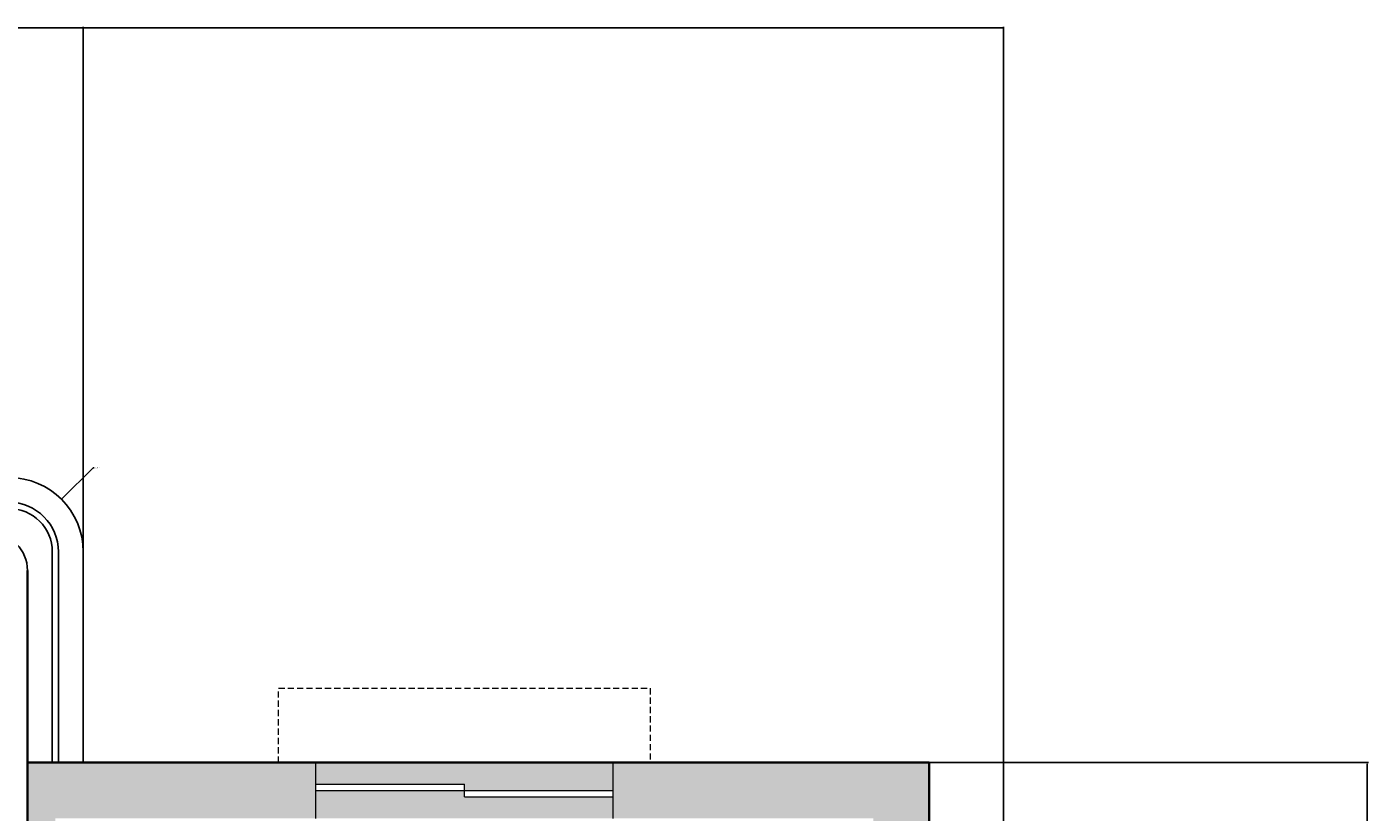
# Model space of a CAD drawing. Units: inches. Extents: x 1693 to 2974, y 2201 to 2965.
# Tile 24 of 24: x 2757 to 2973, y 2838 to 2965. Entities that reach past the tile are written whole.
import ezdxf

# ---------------------------------------------------------------- set-up
doc = ezdxf.new("R2010")
doc.units = ezdxf.units.IN
doc.header["$LTSCALE"] = 2
doc.header["$MEASUREMENT"] = 0
doc.linetypes.add('HIDDEN', pattern=[0.375, 0.25, -0.125])
for name, color, linetype, lineweight in [('A-ANNO-DIMS', 2, 'Continuous', 18), ('A-FLOR-RAIL', 7, 'Continuous', 25), ('A-GLAZ', 4, 'Continuous', 18), ('A-GLAZ-OVHD', 8, 'HIDDEN', 13), ('A-WALL', 7, 'Continuous', 35)]:
    doc.layers.add(name, color=color, linetype=linetype, lineweight=lineweight)
doc.layers.add('A-GLAZ-PATT', color=141, linetype='Continuous', lineweight=13, true_color=0xadddf7)
doc.layers.add('A-WALL-PATT', color=251, linetype='Continuous', lineweight=13, true_color=0x636466)
doc.styles.get("Standard").update_dxf_attribs({"font": 'arial.ttf'})
doc.dimstyles.get("Standard").update_dxf_attribs({"dimtxt": 0.18, "dimasz": 0.18, "dimexe": 0.18, "dimexo": 0.0625, "dimgap": 0.09, "dimtad": 0, "dimtih": 1, "dimtoh": 1, "dimdec": 1, "dimzin": 0, "dimdsep": 46, "dimlunit": 3, "dimtxsty": 'Standard', "dimcen": 0.09, "dimadec": 0, "dimazin": 0, "dimtfac": 1, "dimtdec": 1, "dimtofl": 0, "dimtmove": 0, "dimatfit": 3, "dimfxl": 1, "dimtolj": 1, "dimtzin": 0, "dimarcsym": 0})

# ---------------------------------------------------------------- blocks, each defined once
blk = doc.blocks.new('*D81')
at = {"layer": 'A-ANNO-DIMS', "color": 0, "lineweight": -2, "ltscale": 2, "transparency": 16777216}
for p, q in [((1752.34, 2553.91), (1752.34, 2964.96)), ((1752.52, 2964.78), (2332.94, 2964.78)), ((2914.06, 2964.78), (2333.64, 2964.78)), ((2914.24, 2754.97), (2914.24, 2964.96))]:
    blk.add_line(p, q, dxfattribs=at)
at = {"layer": 'A-ANNO-DIMS', "color": 0, "ltscale": 2, "transparency": 16777216}
for points in [[(1752.52, 2964.81), (1752.52, 2964.75), (1752.34, 2964.78)], [(2914.06, 2964.81), (2914.06, 2964.75), (2914.24, 2964.78)]]:
    blk.add_solid(points, dxfattribs=at)
at = {"layer": 'Defpoints', "color": 0, "ltscale": 2, "transparency": 16777216}
for p in [(2914.24, 2964.78), (2914.24, 2754.9), (1752.34, 2553.84)]:
    blk.add_point(p, dxfattribs=at)
at = {"layer": 'A-ANNO-DIMS', "color": 0, "ltscale": 2, "transparency": 16777216, "insert": (2333.29, 2964.78), "char_height": 0.18, "attachment_point": 5}
blk.add_mtext('\\A1;1162', dxfattribs=at)
blk = doc.blocks.new('*D87')
at = {"layer": 'A-ANNO-DIMS', "color": 0, "lineweight": -2, "ltscale": 2, "transparency": 16777216}
for p, q in [((2902.3, 2846.25), (2973.12, 2846.25)), ((2972.94, 2846.07), (2972.94, 2590.69)), ((2972.94, 2334.93), (2972.94, 2590.32)), ((2902.3, 2334.75), (2973.12, 2334.75))]:
    blk.add_line(p, q, dxfattribs=at)
at = {"layer": 'A-ANNO-DIMS', "color": 0, "ltscale": 2, "transparency": 16777216}
for points in [[(2972.91, 2846.07), (2972.97, 2846.07), (2972.94, 2846.25)], [(2972.91, 2334.93), (2972.97, 2334.93), (2972.94, 2334.75)]]:
    blk.add_solid(points, dxfattribs=at)
at = {"layer": 'Defpoints', "color": 0, "ltscale": 2, "transparency": 16777216}
for p in [(2902.24, 2846.25), (2972.94, 2846.25), (2902.24, 2334.75)]:
    blk.add_point(p, dxfattribs=at)
at = {"layer": 'A-ANNO-DIMS', "color": 0, "ltscale": 2, "transparency": 16777216, "insert": (2972.94, 2590.5), "char_height": 0.18, "attachment_point": 5}
blk.add_mtext('\\A1;511.5', dxfattribs=at)
blk = doc.blocks.new('*D100')
at = {"layer": 'A-ANNO-DIMS', "color": 0, "lineweight": -2, "ltscale": 2, "transparency": 16777216}
for p, q in [((2615.74, 2906.14), (2615.74, 2964.96)), ((2615.92, 2964.78), (2690.46, 2964.78)), ((2765.56, 2964.78), (2691.02, 2964.78)), ((2765.74, 2880.32), (2765.74, 2964.96))]:
    blk.add_line(p, q, dxfattribs=at)
at = {"layer": 'A-ANNO-DIMS', "color": 0, "ltscale": 2, "transparency": 16777216}
for points in [[(2615.92, 2964.81), (2615.92, 2964.75), (2615.74, 2964.78)], [(2765.56, 2964.81), (2765.56, 2964.75), (2765.74, 2964.78)]]:
    blk.add_solid(points, dxfattribs=at)
at = {"layer": 'Defpoints', "color": 0, "ltscale": 2, "transparency": 16777216}
for p in [(2765.74, 2964.78), (2615.74, 2906.08), (2765.74, 2880.25)]:
    blk.add_point(p, dxfattribs=at)
at = {"layer": 'A-ANNO-DIMS', "color": 0, "ltscale": 2, "transparency": 16777216, "insert": (2690.74, 2964.78), "char_height": 0.18, "attachment_point": 5}
blk.add_mtext('\\A1;150', dxfattribs=at)
blk = doc.blocks.new('*D112')
at = {"layer": 'A-ANNO-DIMS', "color": 0, "lineweight": -2, "ltscale": 2, "transparency": 16777216}
for p, q in [((2767.31, 2893.83), (2762.35, 2888.87)), ((2767.49, 2893.83), (2767.31, 2893.83)), ((2753.65, 2880.25), (2753.83, 2880.25)), ((2753.74, 2880.16), (2753.74, 2880.34))]:
    blk.add_line(p, q, dxfattribs=at)
at = {"layer": 'A-ANNO-DIMS', "color": 0, "ltscale": 2, "transparency": 16777216}
blk.add_solid([(2762.33, 2888.89), (2762.37, 2888.85), (2762.22, 2888.74)], dxfattribs=at)
at = {"layer": 'Defpoints', "color": 0, "ltscale": 2, "transparency": 16777216}
for p in [(2762.22, 2888.74), (2753.74, 2880.25)]:
    blk.add_point(p, dxfattribs=at)
at = {"layer": 'A-ANNO-DIMS', "color": 0, "ltscale": 2, "transparency": 16777216, "insert": (2767.99, 2893.83), "char_height": 0.18, "attachment_point": 5}
blk.add_mtext('\\A1;2X R12', dxfattribs=at)

msp = doc.modelspace()

# ---------------------------------------------------------------- hatches: boundary and pattern name
at = {"layer": 'A-GLAZ-PATT', "ltscale": 2}
h = msp.add_hatch(color=256, dxfattribs=at)
h.dxf.hatch_style = 1
h.paths.add_polyline_path([(2656.9702, 2338.2547), (2632.9702, 2338.2547), (2632.9702, 2339.2547), (2608.9702, 2339.2547), (2608.9702, 2334.7547), (2656.9702, 2334.7547)])
h.paths.add_polyline_path([(2656.9702, 2343.7547), (2608.9702, 2343.7547), (2608.9702, 2340.2547), (2632.9702, 2340.2547), (2632.9702, 2339.2547), (2656.9702, 2339.2547)])
h.paths.add_polyline_path([(2775.7544, 2338.2547), (2751.7544, 2338.2547), (2751.7544, 2334.7547), (2775.7544, 2334.7547)])
h.paths.add_polyline_path([(2775.7544, 2343.7547), (2751.7544, 2343.7547), (2751.7544, 2340.2547), (2775.7544, 2340.2547)])
h.paths.add_polyline_path([(2897.7363, 2568.7999), (2893.2363, 2568.7999), (2893.2363, 2520.7999), (2896.7363, 2520.7999), (2896.7363, 2544.7999), (2897.7363, 2544.7999)])
h.paths.add_polyline_path([(2902.2363, 2568.7999), (2898.7363, 2568.7999), (2898.7363, 2544.7999), (2897.7363, 2544.7999), (2897.7363, 2520.7999), (2902.2363, 2520.7999)])
h.paths.add_polyline_path([(2902.2363, 2637.7547), (2898.7363, 2637.7547), (2898.7363, 2613.7547), (2902.2363, 2613.7547)])
h.paths.add_polyline_path([(2896.7363, 2637.7547), (2893.2363, 2637.7547), (2893.2363, 2613.7547), (2896.7363, 2613.7547)])
h.paths.add_polyline_path([(2902.2363, 2748.903), (2899.0477, 2748.903), (2899.0477, 2724.903), (2898.0477, 2724.903), (2898.0477, 2700.903), (2902.2363, 2700.903)])
h.paths.add_polyline_path([(2898.0477, 2748.903), (2893.2363, 2748.903), (2893.2363, 2700.903), (2897.0477, 2700.903), (2897.0477, 2724.903), (2898.0477, 2724.903)])
h.paths.add_polyline_path([(2851.2363, 2846.2547), (2803.2363, 2846.2547), (2803.2363, 2842.7547), (2827.2363, 2842.7547), (2827.2363, 2841.7547), (2851.2363, 2841.7547)])
h.paths.add_polyline_path([(2851.2363, 2840.7547), (2827.2363, 2840.7547), (2827.2363, 2841.7547), (2803.2363, 2841.7547), (2803.2363, 2837.2547), (2851.2363, 2837.2547)])
h.paths.add_polyline_path([(2578.2363, 2846.2547), (2530.2363, 2846.2547), (2530.2363, 2842.7547), (2554.2363, 2842.7547), (2554.2363, 2841.7547), (2578.2363, 2841.7547)])
h.paths.add_polyline_path([(2578.2363, 2840.7547), (2554.2363, 2840.7547), (2554.2363, 2841.7547), (2530.2363, 2841.7547), (2530.2363, 2837.2547), (2578.2363, 2837.2547)])
h.paths.add_polyline_path([(2732.7363, 2812.7547), (2705.1363, 2812.7547), (2705.1363, 2811.7547), (2676.3363, 2811.7547), (2676.3363, 2812.7547), (2648.7363, 2812.7547), (2648.7363, 2808.2547), (2732.7363, 2808.2547)])
h.paths.add_polyline_path([(2732.7363, 2817.2547), (2648.7363, 2817.2547), (2648.7363, 2813.7547), (2676.3363, 2813.7547), (2676.3363, 2812.7547), (2705.1363, 2812.7547), (2705.1363, 2813.7547), (2732.7363, 2813.7547)])
h.paths.add_polyline_path([(2488.2363, 2695.8203), (2484.7878, 2695.8203), (2484.7878, 2671.8203), (2488.2363, 2671.8203)])
h.paths.add_polyline_path([(2482.7878, 2695.8203), (2479.2363, 2695.8203), (2479.2363, 2671.8203), (2482.7878, 2671.8203)])
h.paths.add_polyline_path([(2488.2363, 2572.4371), (2484.7363, 2572.4371), (2484.7363, 2541.4371), (2483.7363, 2541.4371), (2483.7363, 2512.4371), (2488.2363, 2512.4371)])
h.paths.add_polyline_path([(2482.7363, 2541.4371), (2483.7363, 2541.4371), (2483.7363, 2572.4371), (2479.2363, 2572.4371), (2479.2363, 2512.4371), (2482.7363, 2512.4371)])
h.paths.add_polyline_path([(2248.9863, 2706.8449), (2190.9863, 2706.8449), (2190.9863, 2703.3449), (2219.9863, 2703.3449), (2219.9863, 2702.3449), (2248.9863, 2702.3449)])
h.paths.add_polyline_path([(2248.9863, 2701.3449), (2219.9863, 2701.3449), (2219.9863, 2702.3449), (2190.9863, 2702.3449), (2190.9863, 2697.8449), (2248.9863, 2697.8449)])
h.paths.add_polyline_path([(2151.9207, 2293.3449), (2127.9207, 2293.3449), (2127.9207, 2289.8449), (2151.9207, 2289.8449)])
h.paths.add_polyline_path([(2151.9207, 2298.8449), (2127.9207, 2298.8449), (2127.9207, 2295.3449), (2151.9207, 2295.3449)])
h.paths.add_polyline_path([(2084.023, 2293.3449), (2066.023, 2293.3449), (2066.023, 2294.3449), (2048.023, 2294.3449), (2048.023, 2289.8449), (2084.023, 2289.8449)])
h.paths.add_polyline_path([(2084.023, 2298.8449), (2048.023, 2298.8449), (2048.023, 2295.3449), (2066.023, 2295.3449), (2066.023, 2294.3449), (2084.023, 2294.3449)])
h.paths.add_polyline_path([(1966.0781, 2293.3449), (1948.0781, 2293.3449), (1948.0781, 2294.3449), (1930.0781, 2294.3449), (1930.0781, 2289.8449), (1966.0781, 2289.8449)])
h.paths.add_polyline_path([(1966.0781, 2298.8449), (1930.0781, 2298.8449), (1930.0781, 2295.3449), (1948.0781, 2295.3449), (1948.0781, 2294.3449), (1966.0781, 2294.3449)])
h.paths.add_polyline_path([(1787.2363, 2403.1922), (1782.7363, 2403.1922), (1782.7363, 2355.1922), (1786.2363, 2355.1922), (1786.2363, 2379.1922), (1787.2363, 2379.1922)])
h.paths.add_polyline_path([(1791.7363, 2403.1922), (1788.2363, 2403.1922), (1788.2363, 2379.1922), (1787.2363, 2379.1922), (1787.2363, 2355.1922), (1791.7363, 2355.1922)])
h.paths.add_polyline_path([(1786.2363, 2477.5455), (1782.7363, 2477.5455), (1782.7363, 2453.5455), (1786.2363, 2453.5455)])
h.paths.add_polyline_path([(1791.7363, 2477.5455), (1788.2363, 2477.5455), (1788.2363, 2453.5455), (1791.7363, 2453.5455)])
h.paths.add_polyline_path([(1786.2363, 2621.6433), (1782.7363, 2621.6433), (1782.7363, 2585.6433), (1786.2363, 2585.6433)])
h.paths.add_polyline_path([(1791.7363, 2621.6433), (1788.2363, 2621.6433), (1788.2363, 2585.6433), (1791.7363, 2585.6433)])
h.paths.add_polyline_path([(1908.1286, 2706.8449), (1860.1286, 2706.8449), (1860.1286, 2703.3449), (1884.1286, 2703.3449), (1884.1286, 2702.3449), (1908.1286, 2702.3449)])
h.paths.add_polyline_path([(1908.1286, 2701.3449), (1884.1286, 2701.3449), (1884.1286, 2702.3449), (1860.1286, 2702.3449), (1860.1286, 2697.8449), (1908.1286, 2697.8449)])
h.paths.add_polyline_path([(1973.9863, 2706.8449), (1949.9863, 2706.8449), (1949.9863, 2703.3449), (1973.9863, 2703.3449)])
h.paths.add_polyline_path([(1973.9863, 2701.3449), (1949.9863, 2701.3449), (1949.9863, 2697.8449), (1973.9863, 2697.8449)])
h.paths.add_polyline_path([(2112.7363, 2690.3449), (2028.7363, 2690.3449), (2028.7363, 2686.8449), (2056.3363, 2686.8449), (2056.3363, 2685.8449), (2085.1363, 2685.8449), (2085.1363, 2686.8449), (2112.7363, 2686.8449)])
h.paths.add_polyline_path([(2112.7363, 2685.8449), (2085.1363, 2685.8449), (2085.1363, 2684.8449), (2056.3363, 2684.8449), (2056.3363, 2685.8449), (2028.7363, 2685.8449), (2028.7363, 2681.3449), (2112.7363, 2681.3449)])
h.paths.add_polyline_path([(2422.7363, 2640.7547), (2350.7363, 2640.7547), (2350.7363, 2637.2547), (2386.7363, 2637.2547), (2386.7363, 2636.2547), (2422.7363, 2636.2547)])
h.paths.add_polyline_path([(2422.7363, 2635.2547), (2386.7363, 2635.2547), (2386.7363, 2636.2547), (2350.7363, 2636.2547), (2350.7363, 2631.7547), (2422.7363, 2631.7547)])
at = {"layer": 'A-WALL-PATT', "ltscale": 2}
h = msp.add_hatch(color=256, dxfattribs=at)
h.dxf.hatch_style = 1
h.paths.add_polyline_path([(1928.2363, 2733.2161), (1930.9384, 2733.2161), (1930.9384, 2737.2161), (1923.7363, 2737.2161), (1923.7363, 2706.8449), (1908.1286, 2706.8449), (1908.1286, 2697.8449), (1923.7363, 2697.8449), (1923.7363, 2692.8449), (1928.2363, 2692.8449), (1928.2363, 2697.8449), (1949.9863, 2697.8449), (1949.9863, 2706.8449), (1928.2363, 2706.8449)])
h.paths.add_polyline_path([(2004.7363, 2737.2161), (1995.7363, 2737.2161), (1995.7363, 2706.8449), (1985.6374, 2706.8449), (1973.9863, 2706.8449), (1973.9863, 2697.8449), (2000.2363, 2697.8449), (2000.2363, 2686.5348), (2000.3613, 2686.5348), (2000.3613, 2667.0432), (2000.2363, 2601.8449), (1928.2363, 2601.8449), (1928.2363, 2662.8449), (1923.7363, 2662.8449), (1923.7363, 2595.3449), (1928.2363, 2595.3449), (1928.2363, 2597.3449), (2004.7363, 2597.3449), (2004.7363, 2681.3449), (2012.7814, 2681.3449), (2028.7363, 2681.3449), (2028.7363, 2690.3449), (2004.7363, 2690.3449)])
h.paths.add_polyline_path([(2190.9863, 2706.8449), (2184.9863, 2706.8449), (2145.7363, 2706.8449), (2145.7363, 2765.3449), (2145.7363, 2774.5394), (2136.7363, 2774.5394), (2136.7363, 2756.3449), (2136.7363, 2690.3449), (2112.7363, 2690.3449), (2112.7363, 2681.3449), (2136.7363, 2681.3449), (2136.7363, 2597.3449), (2141.2363, 2597.3449), (2141.2363, 2697.8449), (2190.9863, 2697.8449)])
h.paths.add_polyline_path([(1860.1286, 2706.8449), (1782.7363, 2706.8449), (1782.7363, 2621.6433), (1791.7363, 2621.6433), (1791.7363, 2697.8449), (1860.1286, 2697.8449)])
h.paths.add_polyline_path([(1791.7363, 2585.6433), (1782.7363, 2585.6433), (1782.7363, 2562.8449), (1782.7363, 2553.8449), (1752.3363, 2553.8449), (1752.3363, 2544.2586), (1756.3363, 2544.2586), (1756.3363, 2549.3449), (1782.7363, 2549.3449), (1782.7363, 2489.2404), (1782.7363, 2477.5455), (1791.7363, 2477.5455), (1791.7363, 2493.5991), (1791.6113, 2493.5991), (1791.6113, 2513.0907), (1791.6824, 2533.7198, -0.94742783), (1791.7363, 2534.7168), (1791.7363, 2549.3449), (1863.7363, 2549.3449), (1863.7363, 2513.3449), (1866.7363, 2513.3449), (1866.7363, 2549.3449), (1924.7363, 2549.3449), (1924.7363, 2447.3449), (1924.7363, 2442.8449), (1933.7363, 2442.8449), (1933.7363, 2447.3449), (1928.2363, 2447.3449), (1928.2363, 2559.3449), (1923.7363, 2559.3449), (1923.7363, 2553.8449), (1791.7363, 2553.8449), (1791.7363, 2562.8449)])
h.paths.add_polyline_path([(1791.7363, 2442.8449), (1866.7363, 2442.8449), (1866.7363, 2447.3449), (1866.7363, 2483.3449), (1863.7363, 2483.3449), (1863.7363, 2447.3449), (1791.7363, 2447.3449), (1791.7363, 2453.5455), (1782.7363, 2453.5455), (1782.7363, 2447.3449), (1756.3363, 2447.3449), (1756.3363, 2455.7126), (1752.3363, 2455.7126), (1752.3363, 2442.8449), (1782.7363, 2442.8449), (1782.7363, 2403.1922), (1791.7363, 2403.1922)])
h.paths.add_polyline_path([(1930.0781, 2298.8449), (1791.7363, 2298.8449), (1791.7363, 2355.1922), (1782.7363, 2355.1922), (1782.7363, 2289.8449), (1930.0781, 2289.8449)])
h.paths.add_polyline_path([(2624.7363, 2883.2547), (2624.7363, 2902.6165), (2624.7363, 2906.0761), (2615.7363, 2906.0761), (2615.7363, 2892.2547), (2615.7363, 2846.2547), (2578.2363, 2846.2547), (2578.2363, 2837.2547), (2620.2363, 2837.2547), (2620.2363, 2743.2547), (2624.7363, 2743.2547), (2624.7363, 2808.2547), (2648.7363, 2808.2547), (2648.7363, 2817.2547), (2624.7363, 2817.2547)])
h.paths.add_polyline_path([(2530.2363, 2846.2547), (2479.2363, 2846.2547), (2479.2363, 2695.8203), (2488.2363, 2695.8203), (2488.2363, 2700.7547), (2567.2363, 2700.7547), (2567.2363, 2705.2547), (2488.2363, 2705.2547), (2488.2363, 2837.2547), (2530.2363, 2837.2547)])
h.paths.add_polyline_path([(2488.2363, 2487.7547), (2630.2363, 2487.7547, -0.00990191), (2630.2363, 2489.0322), (2630.2363, 2492.2547), (2488.2363, 2492.2547), (2488.2363, 2512.4371), (2479.2363, 2512.4371), (2479.2363, 2334.7547), (2608.9702, 2334.7547), (2608.9702, 2343.7547), (2488.2363, 2343.7547)])
h.paths.add_polyline_path([(2751.7544, 2343.7547), (2672.7363, 2343.7547), (2672.7363, 2409.7547), (2674.7363, 2409.7547), (2674.7363, 2413.7547), (2672.7363, 2413.7547), (2672.7363, 2487.7547), (2732.7363, 2487.7547), (2732.7363, 2413.7547), (2704.7363, 2413.7547), (2704.7363, 2409.7547), (2784.7363, 2409.7547), (2784.7363, 2343.7547), (2775.7544, 2343.7547), (2775.7544, 2334.7547), (2902.2363, 2334.7547), (2902.2363, 2520.7999), (2893.2363, 2520.7999), (2893.2363, 2413.7547), (2856.0145, 2413.7547), (2856.0145, 2409.7547), (2893.2363, 2409.7547), (2893.2363, 2343.7547), (2789.2363, 2343.7547), (2789.2363, 2409.7547), (2819.2363, 2409.7547), (2826.0145, 2409.7547), (2826.0145, 2413.7547), (2789.2363, 2413.7547), (2789.2363, 2492.2547), (2784.7363, 2492.2547), (2784.7363, 2413.7547), (2736.7363, 2413.7547), (2736.7363, 2492.2547), (2672.7363, 2492.2547), (2666.2363, 2492.2547), (2666.2363, 2487.7547), (2668.2363, 2487.7547), (2668.2363, 2343.7547), (2656.9702, 2343.7547), (2656.9702, 2334.7547), (2662.9702, 2334.7547), (2751.7544, 2334.7547)])
h.paths.add_polyline_path([(2902.2363, 2613.7547), (2893.2363, 2613.7547), (2893.2363, 2589.7547), (2785.2363, 2589.7547), (2785.2363, 2661.7547), (2790.2363, 2661.7547), (2790.2363, 2665.2547), (2761.2363, 2665.2547), (2761.2363, 2667.2547), (2756.7363, 2667.2547), (2756.7363, 2661.7547), (2781.2363, 2661.7547), (2781.2363, 2585.7547), (2893.2363, 2585.7547), (2893.2363, 2568.7999), (2902.2363, 2568.7999)])
h.paths.add_polyline_path([(2488.2363, 2671.8203), (2479.2363, 2671.8203), (2479.2363, 2645.2547), (2479.2363, 2623.4598), (2488.2363, 2623.4598), (2488.2363, 2636.2547), (2624.7363, 2636.2547), (2624.7363, 2640.7547), (2603.7363, 2640.7547), (2603.7363, 2700.7547), (2624.7363, 2700.7547), (2624.7363, 2707.2547), (2620.2363, 2707.2547), (2620.2363, 2705.2547), (2597.2363, 2705.2547), (2597.2363, 2700.7547), (2599.2363, 2700.7547), (2599.2363, 2640.7547), (2488.2363, 2640.7547)])
h.paths.add_polyline_path([(2761.2363, 2837.2547), (2803.2363, 2837.2547), (2803.2363, 2846.2547), (2797.2363, 2846.2547), (2765.7363, 2846.2547), (2756.7363, 2846.2547), (2756.7363, 2817.2547), (2732.7363, 2817.2547), (2732.7363, 2808.2547), (2756.7363, 2808.2547), (2756.7363, 2703.2547), (2761.2363, 2703.2547)])
h.paths.add_polyline_path([(2739.7489, 2433.1234), (2786.9181, 2433.1234), (2786.9181, 2455.5122), (2739.7489, 2455.5122)], flags=25)
h = msp.add_hatch(color=256, dxfattribs=at)
h.dxf.hatch_style = 1
h.paths.add_polyline_path([(2902.2363, 2846.2547), (2851.2363, 2846.2547), (2851.2363, 2837.2547), (2893.2363, 2837.2547), (2893.2363, 2748.903), (2902.2363, 2748.903), (2902.2363, 2754.903)])
h.paths.add_polyline_path([(2902.2363, 2700.903), (2893.2363, 2700.903), (2893.2363, 2665.2547), (2817.2363, 2665.2547), (2817.2363, 2661.7547), (2893.2363, 2661.7547), (2893.2363, 2637.7547), (2902.2363, 2637.7547)])

# ---------------------------------------------------------------- linework, layer by layer
at = {"layer": 'A-FLOR-RAIL', "ltscale": 2}
for points in [[(2765.7363, 2846.2547), (2765.7363, 2880.2547, 0.41421356), (2753.7363, 2892.2547), (2624.7363, 2892.2547)], [(2761.7363, 2846.2547), (2761.7363, 2880.2547, 0.41421356), (2753.7363, 2888.2547), (2624.7363, 2888.2547)], [(2760.7363, 2846.2547), (2760.7363, 2880.2547, 0.41421356), (2753.7363, 2887.2547), (2624.7363, 2887.2547)]]:
    msp.add_lwpolyline(points, format="xyb", dxfattribs=at)
msp.add_arc((2750.7363, 2877.2547), 6, 0, 90, dxfattribs=at)
at = {"layer": 'A-GLAZ', "ltscale": 2}
for p, q in [((2803.2363, 2837.2547), (2803.2363, 2846.2547)), ((2851.2363, 2837.2547), (2851.2363, 2846.2547)), ((2803.2363, 2842.7547), (2827.2363, 2842.7547)), ((2827.2363, 2840.7547), (2827.2363, 2842.7547)), ((2803.2363, 2841.7547), (2851.2363, 2841.7547)), ((2827.2363, 2840.7547), (2851.2363, 2840.7547))]:
    msp.add_line(p, q, dxfattribs=at)
at = {"layer": 'A-GLAZ-OVHD', "ltscale": 2}
for p, q in [((2797.2363, 2846.2547), (2797.2363, 2858.2547)), ((2797.2363, 2858.2547), (2851.2363, 2858.2547)), ((2851.2363, 2858.2547), (2857.2363, 2858.2547)), ((2857.2363, 2858.2547), (2857.2363, 2846.2547)), ((2803.2363, 2846.2547), (2797.2363, 2846.2547))]:
    msp.add_line(p, q, dxfattribs=at)
at = {"layer": 'A-WALL'}
for p, q in [((2756.7363, 2877.2547), (2756.7363, 2817.2547)), ((2902.2363, 2846.2547), (2902.2363, 2334.7547))]:
    msp.add_line(p, q, dxfattribs=at)
at = {"layer": 'A-WALL', "ltscale": 2}
for q in [(2756.7363, 2846.2547), (2902.2363, 2846.2547)]:
    msp.add_line((2765.7363, 2846.2547), q, dxfattribs=at)

# ---------------------------------------------------------------- dimensions: what is measured, and where the dimension line sits
at = {"layer": 'A-ANNO-DIMS', "ltscale": 2}
for base, p1, p2, picture, middle in [((2914.2363, 2964.7761), (1752.3363, 2553.8449), (2914.2363, 2754.903), '*D81', (2333.2863, 2964.7761)), ((2765.7363, 2964.7761), (2615.7363, 2906.0761), (2765.7363, 2880.2547), '*D100', (2690.7363, 2964.7761))]:
    dim = msp.add_linear_dim(base=base, p1=p1, p2=p2, dimstyle='Standard', override={"dimdec": 0, "dimlfac": 1, "dimrnd": 0, "dimzin": 0, "dimdsep": 46, "dimlunit": 2}, dxfattribs=at)
    dim.commit()
    dim.dimension.update_dxf_attribs({"geometry": picture, "text_midpoint": middle})
dim = msp.add_radius_dim(center=(2753.7363, 2880.2547), mpoint=(2762.2218, 2888.7398), text='2X <>', dimstyle='Standard', override={"dimdec": 0, "dimlfac": 1, "dimrnd": 0, "dimzin": 0, "dimdsep": 46, "dimlunit": 2}, dxfattribs=at)
dim.commit()
dim.dimension.update_dxf_attribs({"geometry": '*D112', "text_midpoint": (2767.9921, 2893.8308), "dimtype": 164})
dim = msp.add_linear_dim(base=(2972.9363, 2846.2547), p1=(2902.2363, 2334.7547), p2=(2902.2363, 2846.2547), angle=90, dimstyle='Standard', override={"dimdec": 1, "dimlfac": 1, "dimrnd": 0, "dimzin": 0, "dimdsep": 46, "dimlunit": 2}, dxfattribs=at)
dim.commit()
dim.dimension.update_dxf_attribs({"geometry": '*D87', "text_midpoint": (2972.9363, 2590.5047)})

doc.saveas('drawing.dxf')
